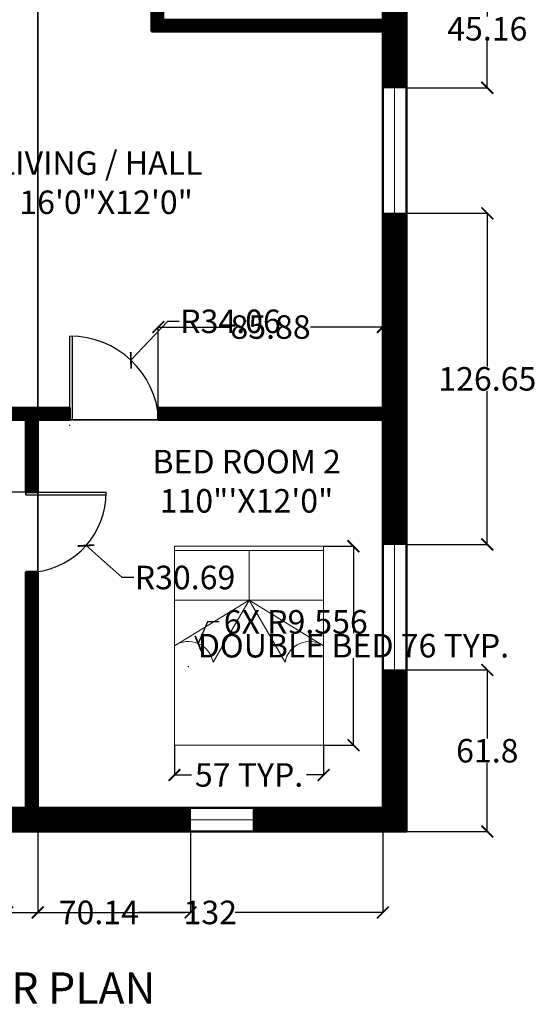
# Model space of a CAD drawing. Units: inches. Extents: x 91 to 526, y 242 to 861.
# Tile 2 of 5: x 328 to 526, y 242 to 618. Entities that reach past the tile are written whole.
import ezdxf

# ---------------------------------------------------------------- set-up
doc = ezdxf.new("R2010")
doc.units = ezdxf.units.IN
doc.header["$MEASUREMENT"] = 0
for name, color, linetype, lineweight in [('A-ANNO-DIMS', 2, 'Continuous', 18), ('A-ANNO-TEXT', 7, 'Continuous', 35), ('A-AREA-IDEN', 7, 'Continuous', 18), ('A-DOOR', 3, 'Continuous', 25), ('A-FURN', 8, 'Continuous', 18), ('A-GLAZ', 4, 'Continuous', 18), ('A-WALL', 7, 'Continuous', 50), ('A-WALL-PATT', 252, 'Continuous', 13)]:
    doc.layers.add(name, color=color, linetype=linetype, lineweight=lineweight)
doc.styles.get("Standard").update_dxf_attribs({"font": 'arial.ttf'})
doc.dimstyles.get("Standard").update_dxf_attribs({"dimtxt": 9, "dimasz": 4.5, "dimexe": 0.18, "dimexo": 0.0625, "dimgap": 0.09, "dimtad": 0, "dimtih": 1, "dimtoh": 1, "dimdec": 1, "dimzin": 0, "dimdsep": 46, "dimlunit": 4, "dimtxsty": 'Standard', "dimblk": 'ARCHTICK', "dimcen": 0.09, "dimadec": 0, "dimazin": 0, "dimtfac": 1, "dimtdec": 1, "dimtofl": 0, "dimtmove": 0, "dimatfit": 3, "dimfxl": 1, "dimtolj": 1, "dimtzin": 0, "dimarcsym": 0})

# ---------------------------------------------------------------- blocks, each defined once
blk = doc.blocks.new('WIN-48')
for p, q in [((0, 9), (48, 9)), ((0, 0), (0, 9)), ((48, 9), (48, 0)), ((0, 4.5), (48, 4.5)), ((48, 0), (0, 0))]:
    blk.add_line(p, q)
blk = doc.blocks.new('WIN-24')
for p, q in [((0, 24), (9, 24)), ((0, 0), (0, 24)), ((4.5, 0), (4.5, 24)), ((9, 24), (9, 0)), ((0, 0), (9, 0))]:
    blk.add_line(p, q)
blk = doc.blocks.new('BED-DOUBLE')
for p, q in [((0, 76.05), (57.04, 76.05)), ((0, 0), (0, 76.05)), ((57.04, 76.05), (57.04, 0)), ((0, 74.47), (57.04, 74.47)), ((28.52, 55.46), (28.52, 74.47)), ((0, 55.46), (57.04, 55.46)), ((28.52, 55.46), (0, 38.03)), ((14.73, 31.74), (28.52, 55.46)), ((57.04, 38.03), (28.52, 55.46)), ((28.52, 55.46), (42.31, 31.74)), ((57.04, 0), (0, 0))]:
    blk.add_line(p, q)
for centre, start, end in [((5.32, 30.09), 9.9572, 123.8152), ((51.72, 30.09), 56.1848, 170.0428)]:
    blk.add_arc(centre, 9.56, start, end)
blk = doc.blocks.new('_ArchTick')
at = {"color": 0, "linetype": 'ByBlock', "const_width": 0.15}
blk.add_lwpolyline([(-0.5, -0.5), (0.5, 0.5)], dxfattribs=at)
blk = doc.blocks.new('*D11')
at = {"layer": 'A-ANNO-DIMS', "color": 0, "lineweight": -2, "transparency": 16777216}
for p, q in [((444.58, 416.76), (456.1, 416.76)), ((455.92, 416.76), (455.92, 383.48)), ((455.92, 340.71), (455.92, 373.99)), ((444.58, 340.71), (456.1, 340.71))]:
    blk.add_line(p, q, dxfattribs=at)
at = {"layer": 'Defpoints', "color": 0, "transparency": 16777216}
for p in [(444.51, 416.76), (455.92, 416.76), (444.51, 340.71)]:
    blk.add_point(p, dxfattribs=at)
at = {"layer": 'A-ANNO-DIMS', "color": 0, "lineweight": -2, "transparency": 16777216, "xscale": 4.5, "yscale": 4.5, "zscale": 4.5}
for p, rotation in [((455.92, 416.76), 90), ((455.92, 340.71), 270)]:
    blk.add_blockref('_ArchTick', p, dxfattribs=dict(at, rotation=rotation))
at = {"layer": 'A-ANNO-DIMS', "color": 0, "transparency": 16777216, "insert": (455.92, 378.74), "char_height": 9, "attachment_point": 5}
blk.add_mtext('\\A1;DOUBLE BED 76 TYP.', dxfattribs=at)
blk = doc.blocks.new('*D12')
at = {"layer": 'A-ANNO-DIMS', "color": 0, "lineweight": -2, "transparency": 16777216}
for p, q in [((387.47, 340.65), (387.47, 329.12)), ((444.51, 340.65), (444.51, 329.12)), ((387.47, 329.3), (394, 329.3)), ((444.51, 329.3), (437.99, 329.3))]:
    blk.add_line(p, q, dxfattribs=at)
at = {"layer": 'Defpoints', "color": 0, "transparency": 16777216}
for p in [(387.47, 340.71), (444.51, 340.71), (444.51, 329.3)]:
    blk.add_point(p, dxfattribs=at)
at = {"layer": 'A-ANNO-DIMS', "color": 0, "lineweight": -2, "transparency": 16777216, "xscale": 4.5, "yscale": 4.5, "zscale": 4.5, "rotation": 180}
blk.add_blockref('_ArchTick', (387.47, 329.3), dxfattribs=at)
at = {"layer": 'A-ANNO-DIMS', "color": 0, "lineweight": -2, "transparency": 16777216, "xscale": 4.5, "yscale": 4.5, "zscale": 4.5}
blk.add_blockref('_ArchTick', (444.51, 329.3), dxfattribs=at)
at = {"layer": 'A-ANNO-DIMS', "color": 0, "transparency": 16777216, "insert": (415.99, 329.3), "char_height": 9, "attachment_point": 5}
blk.add_mtext('\\A1;57 TYP.', dxfattribs=at)
blk = doc.blocks.new('*D25')
at = {"layer": 'A-ANNO-DIMS', "color": 0, "lineweight": -2, "transparency": 16777216}
for p, q in [((323.47, 307.61), (323.47, 276.54)), ((393.61, 307.61), (393.61, 276.54)), ((323.47, 276.72), (343.32, 276.72)), ((393.61, 276.72), (373.76, 276.72))]:
    blk.add_line(p, q, dxfattribs=at)
at = {"layer": 'Defpoints', "color": 0, "transparency": 16777216}
for p in [(323.47, 307.67), (393.61, 307.67), (393.61, 276.72)]:
    blk.add_point(p, dxfattribs=at)
at = {"layer": 'A-ANNO-DIMS', "color": 0, "lineweight": -2, "transparency": 16777216, "xscale": 4.5, "yscale": 4.5, "zscale": 4.5, "rotation": 180}
blk.add_blockref('_ArchTick', (323.47, 276.72), dxfattribs=at)
at = {"layer": 'A-ANNO-DIMS', "color": 0, "lineweight": -2, "transparency": 16777216, "xscale": 4.5, "yscale": 4.5, "zscale": 4.5}
blk.add_blockref('_ArchTick', (393.61, 276.72), dxfattribs=at)
at = {"layer": 'A-ANNO-DIMS', "color": 0, "transparency": 16777216, "insert": (358.54, 276.72), "char_height": 9, "attachment_point": 5}
blk.add_mtext('\\A1;70.14', dxfattribs=at)
blk = doc.blocks.new('*D29')
at = {"layer": 'A-ANNO-DIMS', "color": 0, "lineweight": -2, "transparency": 16777216}
for p, q in [((476.22, 369.48), (507.29, 369.48)), ((507.11, 369.48), (507.11, 343.26)), ((507.11, 307.67), (507.11, 333.89)), ((476.22, 307.67), (507.29, 307.67))]:
    blk.add_line(p, q, dxfattribs=at)
at = {"layer": 'Defpoints', "color": 0, "transparency": 16777216}
for p in [(476.16, 369.48), (507.11, 369.48), (476.16, 307.67)]:
    blk.add_point(p, dxfattribs=at)
at = {"layer": 'A-ANNO-DIMS', "color": 0, "lineweight": -2, "transparency": 16777216, "xscale": 4.5, "yscale": 4.5, "zscale": 4.5}
for p, rotation in [((507.11, 369.48), 90), ((507.11, 307.67), 270)]:
    blk.add_blockref('_ArchTick', p, dxfattribs=dict(at, rotation=rotation))
at = {"layer": 'A-ANNO-DIMS', "color": 0, "transparency": 16777216, "insert": (507.11, 338.57), "char_height": 9, "attachment_point": 5}
blk.add_mtext('\\A1;61.8', dxfattribs=at)
blk = doc.blocks.new('*D30')
at = {"layer": 'A-ANNO-DIMS', "color": 0, "lineweight": -2, "transparency": 16777216}
for p, q in [((476.22, 544.13), (507.29, 544.13)), ((507.11, 544.13), (507.11, 485.49)), ((507.11, 417.48), (507.11, 476.12)), ((476.22, 417.48), (507.29, 417.48))]:
    blk.add_line(p, q, dxfattribs=at)
at = {"layer": 'Defpoints', "color": 0, "transparency": 16777216}
for p in [(476.16, 544.13), (507.11, 544.13), (476.16, 417.48)]:
    blk.add_point(p, dxfattribs=at)
at = {"layer": 'A-ANNO-DIMS', "color": 0, "lineweight": -2, "transparency": 16777216, "xscale": 4.5, "yscale": 4.5, "zscale": 4.5}
for p, rotation in [((507.11, 544.13), 90), ((507.11, 417.48), 270)]:
    blk.add_blockref('_ArchTick', p, dxfattribs=dict(at, rotation=rotation))
at = {"layer": 'A-ANNO-DIMS', "color": 0, "transparency": 16777216, "insert": (507.11, 480.8), "char_height": 9, "attachment_point": 5}
blk.add_mtext('\\A1;126.65', dxfattribs=at)
blk = doc.blocks.new('*D31')
at = {"layer": 'A-ANNO-DIMS', "color": 0, "lineweight": -2, "transparency": 16777216}
for p, q in [((476.22, 637.29), (507.29, 637.29)), ((507.11, 637.29), (507.11, 619.4)), ((507.11, 592.13), (507.11, 610.03)), ((476.22, 592.13), (507.29, 592.13))]:
    blk.add_line(p, q, dxfattribs=at)
at = {"layer": 'Defpoints', "color": 0, "transparency": 16777216}
for p in [(476.16, 637.29), (507.11, 637.29), (476.16, 592.13)]:
    blk.add_point(p, dxfattribs=at)
at = {"layer": 'A-ANNO-DIMS', "color": 0, "lineweight": -2, "transparency": 16777216, "xscale": 4.5, "yscale": 4.5, "zscale": 4.5}
for p, rotation in [((507.11, 637.29), 90), ((507.11, 592.13), 270)]:
    blk.add_blockref('_ArchTick', p, dxfattribs=dict(at, rotation=rotation))
at = {"layer": 'A-ANNO-DIMS', "color": 0, "transparency": 16777216, "insert": (507.11, 614.71), "char_height": 9, "attachment_point": 5}
blk.add_mtext('\\A1;45.16', dxfattribs=at)
blk = doc.blocks.new('*D33')
at = {"layer": 'A-ANNO-DIMS', "color": 0, "lineweight": -2, "transparency": 16777216}
for p, q in [((335.16, 814.61), (335.16, 276.54)), ((467.16, 814.61), (467.16, 276.54)), ((335.16, 276.72), (391.6, 276.72)), ((467.16, 276.72), (410.72, 276.72))]:
    blk.add_line(p, q, dxfattribs=at)
at = {"layer": 'Defpoints', "color": 0, "transparency": 16777216}
for p in [(335.16, 814.67), (467.16, 814.67), (467.16, 276.72)]:
    blk.add_point(p, dxfattribs=at)
at = {"layer": 'A-ANNO-DIMS', "color": 0, "lineweight": -2, "transparency": 16777216, "xscale": 4.5, "yscale": 4.5, "zscale": 4.5, "rotation": 180}
blk.add_blockref('_ArchTick', (335.16, 276.72), dxfattribs=at)
at = {"layer": 'A-ANNO-DIMS', "color": 0, "lineweight": -2, "transparency": 16777216, "xscale": 4.5, "yscale": 4.5, "zscale": 4.5}
blk.add_blockref('_ArchTick', (467.16, 276.72), dxfattribs=at)
at = {"layer": 'A-ANNO-DIMS', "color": 0, "transparency": 16777216, "insert": (401.16, 276.72), "char_height": 9, "attachment_point": 5}
blk.add_mtext('\\A1;132', dxfattribs=at)
blk = doc.blocks.new('*D34')
at = {"layer": 'A-ANNO-DIMS', "color": 0, "lineweight": -2, "transparency": 16777216}
for p, q in [((335.16, 316.73), (335.16, 854.8)), ((335.16, 854.62), (391.6, 854.62)), ((467.16, 854.62), (410.72, 854.62)), ((467.16, 316.73), (467.16, 854.8))]:
    blk.add_line(p, q, dxfattribs=at)
at = {"layer": 'Defpoints', "color": 0, "transparency": 16777216}
for p in [(467.16, 854.62), (335.16, 316.67), (467.16, 316.67)]:
    blk.add_point(p, dxfattribs=at)
at = {"layer": 'A-ANNO-DIMS', "color": 0, "lineweight": -2, "transparency": 16777216, "xscale": 4.5, "yscale": 4.5, "zscale": 4.5, "rotation": 180}
blk.add_blockref('_ArchTick', (335.16, 854.62), dxfattribs=at)
at = {"layer": 'A-ANNO-DIMS', "color": 0, "lineweight": -2, "transparency": 16777216, "xscale": 4.5, "yscale": 4.5, "zscale": 4.5}
blk.add_blockref('_ArchTick', (467.16, 854.62), dxfattribs=at)
at = {"layer": 'A-ANNO-DIMS', "color": 0, "transparency": 16777216, "insert": (401.16, 854.62), "char_height": 9, "attachment_point": 5}
blk.add_mtext('\\A1;132', dxfattribs=at)
blk = doc.blocks.new('*D35')
at = {"layer": 'A-ANNO-DIMS', "color": 0, "lineweight": -2, "transparency": 16777216}
for p, q in [((335.1, 465.17), (304.03, 465.17)), ((304.21, 465.17), (304.21, 395.61)), ((304.21, 316.67), (304.21, 386.24)), ((335.1, 316.67), (304.03, 316.67))]:
    blk.add_line(p, q, dxfattribs=at)
at = {"layer": 'Defpoints', "color": 0, "transparency": 16777216}
for p in [(304.21, 465.17), (335.16, 465.17), (335.16, 316.67)]:
    blk.add_point(p, dxfattribs=at)
at = {"layer": 'A-ANNO-DIMS', "color": 0, "lineweight": -2, "transparency": 16777216, "xscale": 4.5, "yscale": 4.5, "zscale": 4.5}
for p, rotation in [((304.21, 465.17), 90), ((304.21, 316.67), 270)]:
    blk.add_blockref('_ArchTick', p, dxfattribs=dict(at, rotation=rotation))
at = {"layer": 'A-ANNO-DIMS', "color": 0, "transparency": 16777216, "insert": (304.21, 390.92), "char_height": 9, "attachment_point": 5}
blk.add_mtext('\\A1;148.5', dxfattribs=at)
blk = doc.blocks.new('*D50')
at = {"layer": 'A-ANNO-DIMS', "color": 0, "lineweight": -2, "transparency": 16777216}
for p, q in [((330.6, 465.17), (299.53, 465.17)), ((299.71, 465.17), (299.71, 455.97)), ((299.71, 437.4), (299.71, 446.6)), ((330.6, 437.4), (299.53, 437.4))]:
    blk.add_line(p, q, dxfattribs=at)
at = {"layer": 'Defpoints', "color": 0, "transparency": 16777216}
for p in [(299.71, 465.17), (330.66, 465.17), (330.66, 437.4)]:
    blk.add_point(p, dxfattribs=at)
at = {"layer": 'A-ANNO-DIMS', "color": 0, "lineweight": -2, "transparency": 16777216, "xscale": 4.5, "yscale": 4.5, "zscale": 4.5}
for p, rotation in [((299.71, 465.17), 90), ((299.71, 437.4), 270)]:
    blk.add_blockref('_ArchTick', p, dxfattribs=dict(at, rotation=rotation))
at = {"layer": 'A-ANNO-DIMS', "color": 0, "transparency": 16777216, "insert": (299.71, 451.29), "char_height": 9, "attachment_point": 5}
blk.add_mtext('\\A1;27.767', dxfattribs=at)
blk = doc.blocks.new('*D51')
at = {"layer": 'A-ANNO-DIMS', "color": 0, "lineweight": -2, "transparency": 16777216}
for p, q in [((381.28, 469.73), (381.28, 500.8)), ((381.28, 500.62), (408.93, 500.62)), ((467.16, 500.62), (439.51, 500.62)), ((467.16, 469.73), (467.16, 500.8))]:
    blk.add_line(p, q, dxfattribs=at)
at = {"layer": 'Defpoints', "color": 0, "transparency": 16777216}
for p in [(467.16, 500.62), (381.28, 469.67), (467.16, 469.67)]:
    blk.add_point(p, dxfattribs=at)
at = {"layer": 'A-ANNO-DIMS', "color": 0, "lineweight": -2, "transparency": 16777216, "xscale": 4.5, "yscale": 4.5, "zscale": 4.5, "rotation": 180}
blk.add_blockref('_ArchTick', (381.28, 500.62), dxfattribs=at)
at = {"layer": 'A-ANNO-DIMS', "color": 0, "lineweight": -2, "transparency": 16777216, "xscale": 4.5, "yscale": 4.5, "zscale": 4.5}
blk.add_blockref('_ArchTick', (467.16, 500.62), dxfattribs=at)
at = {"layer": 'A-ANNO-DIMS', "color": 0, "transparency": 16777216, "insert": (424.22, 500.62), "char_height": 9, "attachment_point": 5}
blk.add_mtext('\\A1;85.88', dxfattribs=at)
blk = doc.blocks.new('*D60')
at = {"layer": 'A-ANNO-DIMS', "color": 0, "lineweight": -2, "transparency": 16777216}
for p, q in [((384.82, 502.8), (370.81, 487.93)), ((389.32, 502.8), (384.82, 502.8)), ((347.45, 463.04), (347.45, 463.22)), ((347.36, 463.13), (347.54, 463.13))]:
    blk.add_line(p, q, dxfattribs=at)
at = {"layer": 'Defpoints', "color": 0, "transparency": 16777216}
for p in [(370.81, 487.93), (347.45, 463.13)]:
    blk.add_point(p, dxfattribs=at)
at = {"layer": 'A-ANNO-DIMS', "color": 0, "lineweight": -2, "transparency": 16777216, "xscale": 4.5, "yscale": 4.5, "zscale": 4.5, "rotation": 226.7165981565892}
blk.add_blockref('_ArchTick', (370.81, 487.93), dxfattribs=at)
at = {"layer": 'A-ANNO-DIMS', "color": 0, "transparency": 16777216, "insert": (408.9, 502.8), "char_height": 9, "attachment_point": 5}
blk.add_mtext('\\A1;R34.06', dxfattribs=at)
blk = doc.blocks.new('*D62')
at = {"layer": 'A-ANNO-DIMS', "color": 0, "lineweight": -2, "transparency": 16777216}
for p, q in [((330.57, 437.4), (330.75, 437.4)), ((330.66, 437.31), (330.66, 437.49)), ((367.41, 404.83), (353.63, 417.04)), ((371.91, 404.83), (367.41, 404.83))]:
    blk.add_line(p, q, dxfattribs=at)
at = {"layer": 'Defpoints', "color": 0, "transparency": 16777216}
for p in [(330.66, 437.4), (353.63, 417.04)]:
    blk.add_point(p, dxfattribs=at)
at = {"layer": 'A-ANNO-DIMS', "color": 0, "lineweight": -2, "transparency": 16777216, "xscale": 4.5, "yscale": 4.5, "zscale": 4.5, "rotation": 138.4450052505623}
blk.add_blockref('_ArchTick', (353.63, 417.04), dxfattribs=at)
at = {"layer": 'A-ANNO-DIMS', "color": 0, "transparency": 16777216, "insert": (391.5, 404.83), "char_height": 9, "attachment_point": 5}
blk.add_mtext('\\A1;R30.69', dxfattribs=at)
blk = doc.blocks.new('*D67')
at = {"layer": 'A-ANNO-DIMS', "color": 0, "lineweight": -2, "transparency": 16777216}
for p, q in [((400.08, 387.86), (396.54, 379.59)), ((404.58, 387.86), (400.08, 387.86)), ((392.7, 370.8), (392.88, 370.8)), ((392.79, 370.71), (392.79, 370.89))]:
    blk.add_line(p, q, dxfattribs=at)
at = {"layer": 'Defpoints', "color": 0, "transparency": 16777216}
for p in [(396.54, 379.59), (392.79, 370.8)]:
    blk.add_point(p, dxfattribs=at)
at = {"layer": 'A-ANNO-DIMS', "color": 0, "lineweight": -2, "transparency": 16777216, "xscale": 4.5, "yscale": 4.5, "zscale": 4.5, "rotation": 246.8828193868354}
blk.add_blockref('_ArchTick', (396.54, 379.59), dxfattribs=at)
at = {"layer": 'A-ANNO-DIMS', "color": 0, "transparency": 16777216, "insert": (433.85, 387.86), "char_height": 9, "attachment_point": 5}
blk.add_mtext('\\A1;6X R9.556', dxfattribs=at)

msp = doc.modelspace()

# ---------------------------------------------------------------- hatches: boundary and pattern name
at = {"layer": 'A-WALL-PATT'}
h = msp.add_hatch(dxfattribs=at)
h.set_pattern_fill('ANSI31', color=256)
h.paths.add_polyline_path([(476.1605, 544.131), (467.1605, 544.131), (467.1605, 469.6714), (381.2784, 469.6714), (381.2784, 467.1295, -0.01443214), (381.4527, 465.1714), (467.1605, 465.1714), (467.1605, 417.4774), (476.1605, 417.4774)])
h.paths.add_polyline_path([(476.1605, 637.294), (467.1605, 637.294), (467.1605, 618.1714), (383.1605, 618.1714), (383.1605, 650.6481), (381.8098, 650.6481, -0.04281846), (378.6605, 650.378), (378.6605, 618.1714), (378.6605, 613.6714), (467.1605, 613.6714), (467.1605, 592.131), (476.1605, 592.131)])
h.paths.add_polyline_path([(476.1605, 699.6337), (467.1605, 699.6337), (467.1605, 682.6714), (378.6605, 682.6714), (367.8126, 682.6714), (367.8126, 678.1714), (378.6605, 678.1714), (378.6605, 668.8665), (383.1605, 668.8665), (383.1605, 678.1714), (467.1605, 678.1714), (467.1605, 661.294), (476.1605, 661.294)])
h.paths.add_polyline_path([(476.1605, 823.6714), (423.2305, 823.6714), (423.2305, 814.6714), (467.1605, 814.6714), (467.1605, 747.6337), (476.1605, 747.6337)])
h.paths.add_polyline_path([(375.2305, 823.6714), (311.1029, 823.6714), (311.1029, 814.6714), (330.6605, 814.6714), (330.6605, 682.6714), (335.1605, 682.6714), (335.1605, 814.6714), (375.2305, 814.6714)])
h.paths.add_polyline_path([(287.1029, 823.6714), (230.7133, 823.6714), (230.7133, 814.6714), (266.1605, 814.6714), (266.1605, 755.4247), (270.6605, 755.4247), (270.6605, 814.6714), (287.1029, 814.6714)])
h.paths.add_polyline_path([(182.7133, 823.6714), (137.1605, 823.6714), (137.1605, 675.6513), (146.1605, 675.6513), (146.1605, 714.1714), (178.4758, 714.1714), (178.4758, 718.6714), (146.1605, 718.6714), (146.1605, 814.6714), (182.7133, 814.6714)])
h.paths.add_polyline_path([(146.1605, 577.6714), (206.1605, 577.6714), (206.1605, 557.5953), (210.6605, 557.5953), (210.6605, 577.6714), (233.4933, 577.6714), (233.4933, 582.1714), (210.6605, 582.1714), (146.1605, 582.1714), (146.1605, 627.6513), (137.1605, 627.6513), (137.1605, 508.0167), (146.1605, 508.0167), (146.1605, 525.1714), (210.6605, 525.1714), (233.4933, 525.1714), (233.4933, 529.6714), (210.6605, 529.6714), (210.6605, 536.5826), (206.1605, 536.5826), (206.1605, 529.6714), (146.1605, 529.6714)])
h.paths.add_polyline_path([(146.1605, 460.0167), (137.1605, 460.0167), (137.1605, 360.2935), (146.1605, 360.2935), (146.1605, 376.6714), (210.6605, 376.6714), (213.2441, 376.6714, -0.02418169), (213.3544, 378.9513), (213.3544, 381.1714), (210.6605, 381.1714), (146.1605, 381.1714)])
h.paths.add_polyline_path([(146.1605, 336.2935), (137.1605, 336.2935), (137.1605, 307.6714), (146.1605, 307.6714), (177.3362, 307.6714), (177.3362, 316.6714), (146.1605, 316.6714)])
h.paths.add_polyline_path([(393.6086, 316.6714), (323.4726, 316.6714), (323.4726, 307.6714), (393.6086, 307.6714)])
h.paths.add_polyline_path([(256.39, 316.6714), (201.3362, 316.6714), (201.3362, 307.6714), (256.39, 307.6714)])
h.paths.add_polyline_path([(246.6605, 376.6714), (246.6605, 381.1714), (236.8559, 381.1714), (236.8559, 376.6714), (242.1605, 376.6714), (242.1605, 316.6714), (246.6605, 316.6714)])
h = msp.add_hatch(dxfattribs=at)
h.set_pattern_fill('ANSI31', color=256)
h.paths.add_polyline_path([(476.1605, 369.4774), (467.1605, 369.4774), (467.1605, 316.6714), (417.6086, 316.6714), (417.6086, 307.6714), (476.1605, 307.6714)])
h.paths.add_polyline_path([(330.6605, 718.6714), (270.6605, 718.6714), (270.6605, 730.9304), (266.1605, 730.9304), (266.1605, 718.6714), (266.1605, 714.1714), (270.6605, 714.1714), (330.6605, 714.1714)])
h = msp.add_hatch(dxfattribs=at)
h.set_pattern_fill('ANSI31', color=256)
h.paths.add_polyline_path([(335.1605, 465.1714), (347.4545, 465.1714), (347.4545, 469.6714), (335.1605, 469.6714), (330.6605, 469.6714), (275.1605, 469.6714), (275.1605, 613.6714), (270.6605, 613.6714), (270.6605, 469.6714), (270.6605, 465.1714), (290.1605, 465.1714), (290.1605, 381.1714), (281.6979, 381.1714), (281.6979, 376.6714), (294.6605, 376.6714), (294.6605, 381.1714), (294.6605, 465.1714), (330.6605, 465.1714), (330.6605, 437.4043), (335.1605, 437.4043)])
h = msp.add_hatch(dxfattribs=at)
h.set_pattern_fill('ANSI31', color=256)
h.paths.add_polyline_path([(335.1605, 406.9337), (330.6605, 406.9337), (330.6605, 316.6714), (335.1605, 316.6714)])

# ---------------------------------------------------------------- linework, layer by layer
at = {"layer": 'A-DOOR'}
for p, q in [((347.4545, 465.1714), (347.4545, 497.1919)), ((348.4545, 465.1714), (348.4545, 497.1772)), ((347.4545, 465.1714), (381.4527, 465.1714)), ((381.4527, 465.1714), (347.4545, 465.1714)), ((330.6605, 437.4043), (330.6605, 436.4043)), ((330.6605, 436.4043), (330.6605, 437.4043)), ((330.6605, 437.4043), (361.3528, 437.4043)), ((330.6605, 436.4043), (361.3365, 436.4043))]:
    msp.add_line(p, q, dxfattribs=at)
for centre, radius, start, end in [((347.4545, 463.1327), 34.0592, 3.431784, 90), ((330.6605, 437.4043), 30.6923, 276.890247, 0)]:
    msp.add_arc(centre, radius, start, end, dxfattribs=at)
at = {"layer": 'A-WALL'}
for p, q in [((476.1605, 823.6714), (476.1605, 307.6714)), ((467.1605, 678.1714), (467.1605, 618.1714)), ((378.6605, 650.6481), (378.6605, 618.1714)), ((383.1605, 650.6481), (383.1605, 618.1714)), ((378.6605, 618.1714), (378.6605, 613.6714)), ((383.1605, 618.1714), (467.1605, 618.1714)), ((378.6605, 613.6714), (467.1605, 613.6714)), ((467.1605, 613.6714), (467.1605, 469.6714)), ((330.6605, 469.6714), (275.1605, 469.6714)), ((335.1605, 469.6714), (330.6605, 469.6714)), ((335.1605, 469.6714), (347.4545, 469.6714)), ((347.4545, 469.6714), (347.4545, 465.1714)), ((381.2784, 469.6714), (381.2784, 465.1714)), ((381.2784, 469.6714), (467.1605, 469.6714)), ((330.6605, 465.1714), (294.6605, 465.1714)), ((330.6605, 465.1714), (330.6605, 437.4043)), ((335.1605, 465.1714), (347.4545, 465.1714)), ((335.1605, 465.1714), (335.1605, 437.4043)), ((381.2784, 465.1714), (467.1605, 465.1714)), ((467.1605, 465.1714), (467.1605, 316.6714)), ((330.6605, 437.4043), (335.1605, 437.4043)), ((330.6605, 406.9337), (335.1605, 406.9337)), ((330.6605, 406.9337), (330.6605, 307.6714)), ((335.1605, 406.9337), (335.1605, 316.6714)), ((266.1605, 316.6714), (467.1605, 316.6714)), ((266.1605, 307.6714), (476.1605, 307.6714))]:
    msp.add_line(p, q, dxfattribs=at)

# ---------------------------------------------------------------- block references
at = {"layer": 'A-FURN'}
msp.add_blockref('BED-DOUBLE', (387.4737, 340.7098), dxfattribs=at)
at = {"layer": 'A-GLAZ'}
for name, p, rotation in [('WIN-48', (467.1601, 592.1313), 270.0000000000003), ('WIN-48', (467.1601, 417.4777), 270.0000000000003), ('WIN-24', (417.6091, 307.6719), 90.0000000000003)]:
    msp.add_blockref(name, p, dxfattribs=dict(at, rotation=rotation))

# ---------------------------------------------------------------- texts
at = {"layer": 'A-ANNO-TEXT', "insert": (199.4792, 253.7956), "char_height": 12, "attachment_point": 1}
msp.add_mtext_dynamic_manual_height_columns('   GROUND FLOOR PLAN', width=594.11726, gutter_width=1, heights=[0], dxfattribs=at)
at = {"layer": 'A-AREA-IDEN', "char_height": 9, "attachment_point": 1}
for s, insert in [('LIVING / HALL\\P   16\'0"X12\'0"', (319.8733, 567.8393)), ('BED ROOM 2\\P 110"\'X12\'0"', (379.0597, 453.6483))]:
    msp.add_mtext_dynamic_manual_height_columns(s, width=356.121763, gutter_width=1, heights=[0], dxfattribs=dict(at, insert=insert))

# ---------------------------------------------------------------- dimensions: what is measured, and where the dimension line sits
at = {"layer": 'A-ANNO-DIMS'}
for base, p1, p2, override, picture, middle in [((467.1605, 854.6214), (335.1605, 316.6714), (467.1605, 316.6714), {"dimdec": 0, "dimlfac": 1, "dimrnd": 0, "dimzin": 0, "dimdsep": 46, "dimlunit": 2}, '*D34', (401.1605, 854.6214)), ((467.1605, 276.7214), (335.1605, 814.6714), (467.1605, 814.6714), {"dimdec": 0, "dimlfac": 1, "dimrnd": 0, "dimzin": 0, "dimdsep": 46, "dimlunit": 2}, '*D33', (401.1605, 276.7214)), ((467.1605, 500.6214), (381.2784, 469.6714), (467.1605, 469.6714), {"dimdec": 2, "dimlfac": 1, "dimrnd": 0, "dimzin": 0, "dimdsep": 46, "dimlunit": 2}, '*D51', (424.2195, 500.6214)), ((393.6086, 276.7214), (323.4726, 307.6714), (393.6086, 307.6714), {"dimdec": 2, "dimlfac": 1, "dimrnd": 0, "dimzin": 0, "dimdsep": 46, "dimlunit": 2}, '*D25', (358.5406, 276.7214))]:
    dim = msp.add_linear_dim(base=base, p1=p1, p2=p2, dimstyle='Standard', override=override, dxfattribs=at)
    dim.commit()
    dim.dimension.update_dxf_attribs({"geometry": picture, "text_midpoint": middle})
for base, p1, p2, override, picture, middle in [((507.1105, 637.294), (476.1605, 592.131), (476.1605, 637.294), {"dimdec": 2, "dimlfac": 1, "dimrnd": 0, "dimzin": 0, "dimdsep": 46, "dimlunit": 2}, '*D31', (507.1105, 614.7125)), ((507.1105, 544.131), (476.1605, 417.4774), (476.1605, 544.131), {"dimdec": 2, "dimlfac": 1, "dimrnd": 0, "dimzin": 0, "dimdsep": 46, "dimlunit": 2}, '*D30', (507.1105, 480.8042)), ((299.7105, 465.1714), (330.6605, 437.4043), (330.6605, 465.1714), {"dimdec": 3, "dimlfac": 1, "dimrnd": 0, "dimzin": 0, "dimdsep": 46, "dimlunit": 2}, '*D50', (299.7105, 451.2878)), ((304.2105, 465.1714), (335.1605, 316.6714), (335.1605, 465.1714), {"dimdec": 1, "dimlfac": 1, "dimrnd": 0, "dimzin": 0, "dimdsep": 46, "dimlunit": 2}, '*D35', (304.2105, 390.9214)), ((507.1105, 369.4774), (476.1605, 307.6714), (476.1605, 369.4774), {"dimdec": 1, "dimlfac": 1, "dimrnd": 0, "dimzin": 0, "dimdsep": 46, "dimlunit": 2}, '*D29', (507.1105, 338.5744))]:
    dim = msp.add_linear_dim(base=base, p1=p1, p2=p2, angle=90, dimstyle='Standard', override=override, dxfattribs=at)
    dim.commit()
    dim.dimension.update_dxf_attribs({"geometry": picture, "text_midpoint": middle})
for center, mpoint, picture, middle in [((347.4545, 463.1327), (370.8058, 487.9268), '*D60', (408.8953, 502.8033)), ((330.6605, 437.4043), (353.6281, 417.0449), '*D62', (391.4997, 404.8293))]:
    dim = msp.add_radius_dim(center=center, mpoint=mpoint, dimstyle='Standard', override={"dimdec": 2, "dimlfac": 1, "dimrnd": 0, "dimzin": 0, "dimdsep": 46, "dimlunit": 2}, dxfattribs=at)
    dim.commit()
    dim.dimension.update_dxf_attribs({"geometry": picture, "text_midpoint": middle, "dimtype": 164})
dim = msp.add_linear_dim(base=(455.921, 416.7626), p1=(444.513, 340.7095), p2=(444.513, 416.7626), angle=90, text='DOUBLE BED <> TYP.', dimstyle='Standard', override={"dimdec": 0, "dimlfac": 1, "dimrnd": 0, "dimzin": 0, "dimdsep": 46, "dimlunit": 2}, dxfattribs=at)
dim.commit()
dim.dimension.update_dxf_attribs({"geometry": '*D11', "text_midpoint": (455.921, 378.7361)})
dim = msp.add_radius_dim(center=(392.7913, 370.7966), mpoint=(396.5431, 379.5853), text='6X <>', dimstyle='Standard', override={"dimdec": 3, "dimlfac": 1, "dimrnd": 0, "dimzin": 0, "dimdsep": 46, "dimlunit": 2}, dxfattribs=at)
dim.commit()
dim.dimension.update_dxf_attribs({"geometry": '*D67', "text_midpoint": (433.8491, 387.8626)})
dim = msp.add_linear_dim(base=(444.513, 329.3016), p1=(387.4732, 340.7095), p2=(444.513, 340.7095), text='<> TYP.', dimstyle='Standard', override={"dimdec": 0, "dimlfac": 1, "dimrnd": 0, "dimzin": 0, "dimdsep": 46, "dimlunit": 2}, dxfattribs=at)
dim.commit()
dim.dimension.update_dxf_attribs({"geometry": '*D12', "text_midpoint": (415.9931, 329.3016)})

doc.saveas('drawing.dxf')
